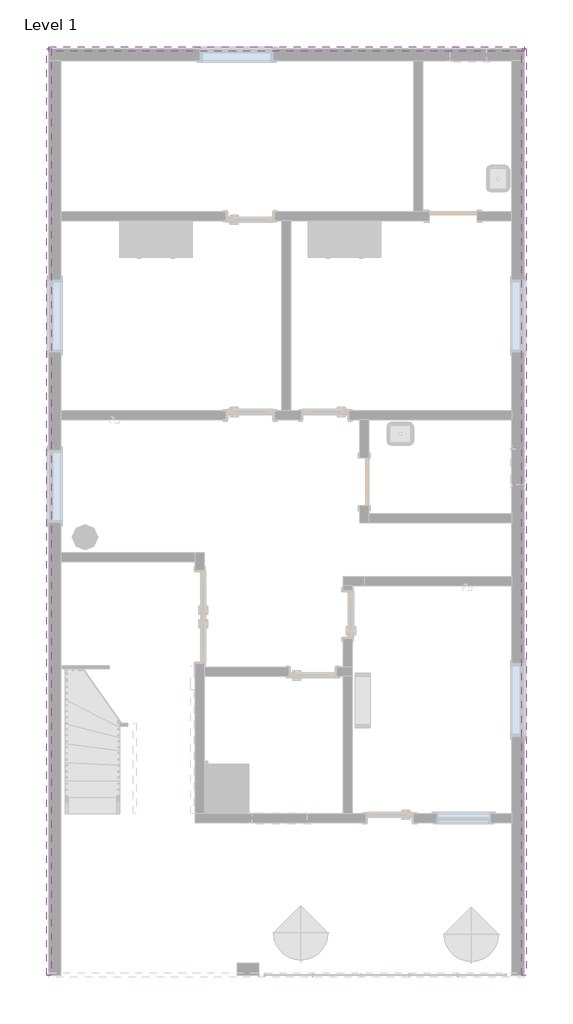
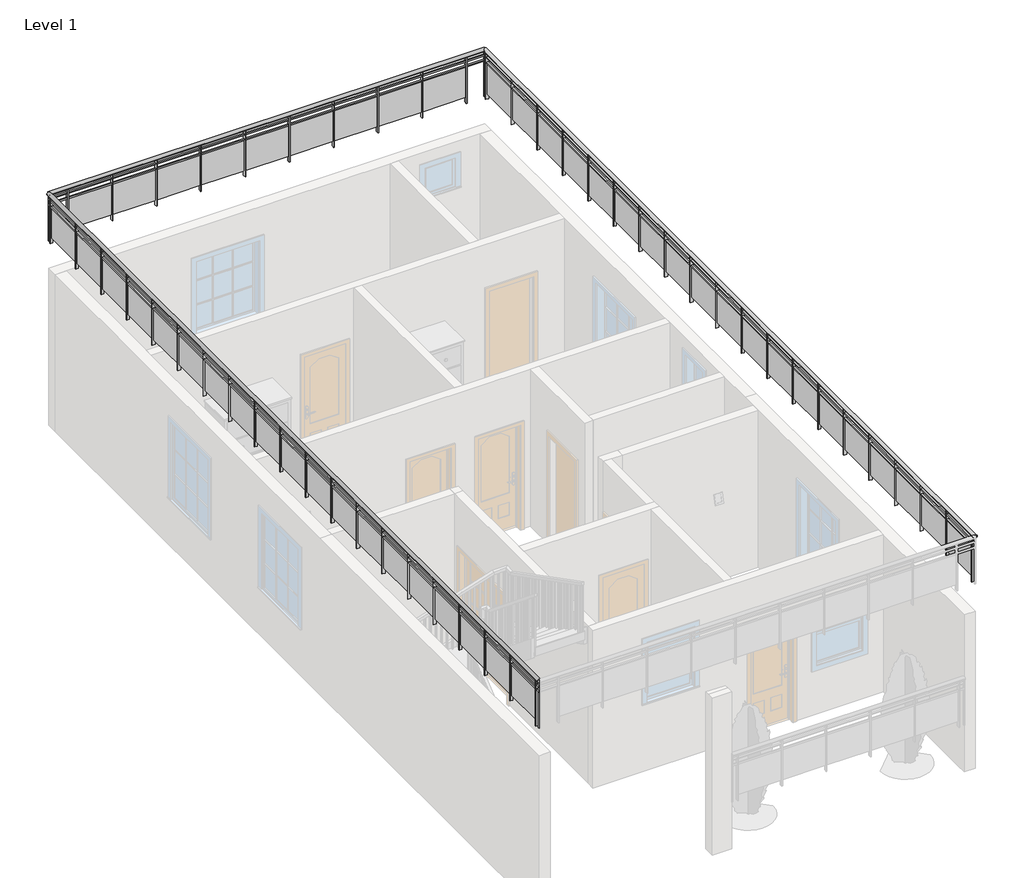
# One storey, part 3 of 4: 3 railings.
"""IFC4 building model written with IfcOpenShell, lengths in millimetres."""

from ifc_helpers import new_model, si_unit, point, frame, origin, place, context, project, spatial, polyline, ellipse_curve, trimmed, outline, extrude, element, save
from ifc_brep_helpers import plane_surface, extruded_surface, advanced_brep

model = new_model("IFC4")

# Units and contexts
model_context = context("Model", 3, world=origin())
ifc_project = project(units=[si_unit("LENGTHUNIT", "METRE", prefix="MILLI")], contexts=[model_context])

# Site, building, storey
site = spatial("IfcSite", under=ifc_project)
building = spatial("IfcBuilding", under=site)
storey = spatial("IfcBuildingStorey", under=building, Name="Level 1", Elevation=0.0)

# Railings
placement = place(None, origin())
element("IfcRailing", 1, ObjectType="Glass Panel - Bottom Fill", at=placement, inside=storey, context=model_context, shape_type="SolidModel", body=[
    advanced_brep(
    [(-13526.4568901, 13670.121124, 4495.8), (-13602.6568901, 13670.121124, 4495.8), (-13526.4568901, -1925.478876, 4495.8), (-13602.6568901, -1925.478876, 4495.8)],
    [
        (0, 1, ellipse_curve(frame((-13564.5568901, 13670.121124, 4495.8), z_axis=(0.0, 1.0, 0.0), x_axis=(-1.0, 0.0, 0.0)), 38.1, 28.575)),
        (1, 0, ellipse_curve(frame((-13564.5568901, 13670.121124, 4495.8), z_axis=(0.0, 1.0, 0.0), x_axis=(-1.0, 0.0, 0.0)), 38.1, 28.575)),
        (2, 3, ellipse_curve(frame((-13564.5568901, -1925.478876, 4495.8), z_axis=(0.0, -1.0, 0.0), x_axis=(-1.0, 0.0, 0.0)), 38.1, 28.575)),
        (3, 2, ellipse_curve(frame((-13564.5568901, -1925.478876, 4495.8), z_axis=(0.0, -1.0, 0.0), x_axis=(-1.0, 0.0, 0.0)), 38.1, 28.575)),
        (0, 2),
        (3, 1),
    ],
    [
        plane_surface(frame((-13564.5568901, 13670.121124, 4495.8), z_axis=(0.0, 1.0, 0.0), x_axis=(0.0, 0.0, -1.0))),
        plane_surface(frame((-13564.5568901, -1925.478876, 4495.8), z_axis=(0.0, -1.0, 0.0), x_axis=(0.0, 0.0, -1.0))),
        extruded_surface(trimmed(ellipse_curve(frame((-13564.5568901, -1925.478876, 4495.8), z_axis=(0.0, 1.0, 0.0), x_axis=(-1.0, 0.0, 0.0)), 38.1, 28.575), [point((-13526.4568901, -1925.478876, 4495.8))], [point((-13602.6568901, -1925.478876, 4495.8))], True, "CARTESIAN"), (0.0, 15595.599999999999, 0.0), 15595.599999999999),
        extruded_surface(trimmed(ellipse_curve(frame((-13564.5568901, -1925.478876, 4495.8), z_axis=(0.0, 1.0, 0.0), x_axis=(-1.0, 0.0, 0.0)), 38.1, 28.575), [point((-13602.6568901, -1925.478876, 4495.8))], [point((-13526.4568901, -1925.478876, 4495.8))], True, "CARTESIAN"), (0.0, 15595.599999999999, 0.0), 15595.599999999999),
    ],
    [
        (0, [[1, 2]]),
        (1, [[3, 4]]),
        (2, [[-1, 5, -4, 6]]),
        (3, [[-2, -6, -3, -5]]),
    ],
),
    extrude(outline(polyline([(-13577.2568901, 13670.121124), (-13551.8568901, 13670.121124), (-13551.8568901, -1925.478876), (-13577.2568901, -1925.478876), (-13577.2568901, 13670.121124)])), frame((0.0, 0.0, 4381.5), z_axis=(0.0, 0.0, 1.0), x_axis=(1.0, 0.0, 0.0)), (0.0, 0.0, 1.0), 25.4),
    extrude(outline(polyline([(-13577.2568901, 13670.121124), (-13551.8568901, 13670.121124), (-13551.8568901, -1925.478876), (-13577.2568901, -1925.478876), (-13577.2568901, 13670.121124)])), frame((0.0, 0.0, 4279.9), z_axis=(0.0, 0.0, 1.0), x_axis=(1.0, 0.0, 0.0)), (0.0, 0.0, 1.0), 25.4),
    extrude(outline(polyline([(-13589.9568901, -1842.928876), (-13539.1568901, -1842.928876), (-13539.1568901, -1855.628876), (-13589.9568901, -1855.628876), (-13589.9568901, -1842.928876)])), frame((0.0, 0.0, 3581.4), z_axis=(0.0, 0.0, 1.0), x_axis=(1.0, 0.0, 0.0)), (0.0, 0.0, 1.0), 885.6788223),
    extrude(outline(polyline([(-13558.0217331, -1036.478876), (-13558.0217331, -1849.278876), (-13564.3717331, -1849.278876), (-13564.3717331, -1036.478876), (-13558.0217331, -1036.478876)])), frame((0.0, 0.0, 3683.0), z_axis=(0.0, 0.0, 1.0), x_axis=(1.0, 0.0, 0.0)), (0.0, 0.0, 1.0), 596.9),
    extrude(outline(polyline([(-13589.9568901, -1030.128876), (-13539.1568901, -1030.128876), (-13539.1568901, -1042.828876), (-13589.9568901, -1042.828876), (-13589.9568901, -1030.128876)])), frame((0.0, 0.0, 3581.4), z_axis=(0.0, 0.0, 1.0), x_axis=(1.0, 0.0, 0.0)), (0.0, 0.0, 1.0), 885.6788223),
    extrude(outline(polyline([(-13558.0217331, -223.678876), (-13558.0217331, -1036.478876), (-13564.3717331, -1036.478876), (-13564.3717331, -223.678876), (-13558.0217331, -223.678876)])), frame((0.0, 0.0, 3683.0), z_axis=(0.0, 0.0, 1.0), x_axis=(1.0, 0.0, 0.0)), (0.0, 0.0, 1.0), 596.9),
    extrude(outline(polyline([(-13589.9568901, -217.328876), (-13539.1568901, -217.328876), (-13539.1568901, -230.028876), (-13589.9568901, -230.028876), (-13589.9568901, -217.328876)])), frame((0.0, 0.0, 3581.4), z_axis=(0.0, 0.0, 1.0), x_axis=(1.0, 0.0, 0.0)), (0.0, 0.0, 1.0), 885.6788223),
    extrude(outline(polyline([(-13558.0217331, 589.121124), (-13558.0217331, -223.678876), (-13564.3717331, -223.678876), (-13564.3717331, 589.121124), (-13558.0217331, 589.121124)])), frame((0.0, 0.0, 3683.0), z_axis=(0.0, 0.0, 1.0), x_axis=(1.0, 0.0, 0.0)), (0.0, 0.0, 1.0), 596.9),
    extrude(outline(polyline([(-13589.9568901, 595.471124), (-13539.1568901, 595.471124), (-13539.1568901, 582.771124), (-13589.9568901, 582.771124), (-13589.9568901, 595.471124)])), frame((0.0, 0.0, 3581.4), z_axis=(0.0, 0.0, 1.0), x_axis=(1.0, 0.0, 0.0)), (0.0, 0.0, 1.0), 885.6788223),
    extrude(outline(polyline([(-13558.0217331, 1401.921124), (-13558.0217331, 589.121124), (-13564.3717331, 589.121124), (-13564.3717331, 1401.921124), (-13558.0217331, 1401.921124)])), frame((0.0, 0.0, 3683.0), z_axis=(0.0, 0.0, 1.0), x_axis=(1.0, 0.0, 0.0)), (0.0, 0.0, 1.0), 596.9),
    extrude(outline(polyline([(-13589.9568901, 1408.271124), (-13539.1568901, 1408.271124), (-13539.1568901, 1395.571124), (-13589.9568901, 1395.571124), (-13589.9568901, 1408.271124)])), frame((0.0, 0.0, 3581.4), z_axis=(0.0, 0.0, 1.0), x_axis=(1.0, 0.0, 0.0)), (0.0, 0.0, 1.0), 885.6788223),
    extrude(outline(polyline([(-13558.0217331, 2214.721124), (-13558.0217331, 1401.921124), (-13564.3717331, 1401.921124), (-13564.3717331, 2214.721124), (-13558.0217331, 2214.721124)])), frame((0.0, 0.0, 3683.0), z_axis=(0.0, 0.0, 1.0), x_axis=(1.0, 0.0, 0.0)), (0.0, 0.0, 1.0), 596.9),
    extrude(outline(polyline([(-13589.9568901, 2221.071124), (-13539.1568901, 2221.071124), (-13539.1568901, 2208.371124), (-13589.9568901, 2208.371124), (-13589.9568901, 2221.071124)])), frame((0.0, 0.0, 3581.4), z_axis=(0.0, 0.0, 1.0), x_axis=(1.0, 0.0, 0.0)), (0.0, 0.0, 1.0), 885.6788223),
    extrude(outline(polyline([(-13558.0217331, 3027.521124), (-13558.0217331, 2214.721124), (-13564.3717331, 2214.721124), (-13564.3717331, 3027.521124), (-13558.0217331, 3027.521124)])), frame((0.0, 0.0, 3683.0), z_axis=(0.0, 0.0, 1.0), x_axis=(1.0, 0.0, 0.0)), (0.0, 0.0, 1.0), 596.9),
    extrude(outline(polyline([(-13589.9568901, 3033.871124), (-13539.1568901, 3033.871124), (-13539.1568901, 3021.171124), (-13589.9568901, 3021.171124), (-13589.9568901, 3033.871124)])), frame((0.0, 0.0, 3581.4), z_axis=(0.0, 0.0, 1.0), x_axis=(1.0, 0.0, 0.0)), (0.0, 0.0, 1.0), 885.6788223),
    extrude(outline(polyline([(-13558.0217331, 3840.321124), (-13558.0217331, 3027.521124), (-13564.3717331, 3027.521124), (-13564.3717331, 3840.321124), (-13558.0217331, 3840.321124)])), frame((0.0, 0.0, 3683.0), z_axis=(0.0, 0.0, 1.0), x_axis=(1.0, 0.0, 0.0)), (0.0, 0.0, 1.0), 596.9),
    extrude(outline(polyline([(-13589.9568901, 3846.671124), (-13539.1568901, 3846.671124), (-13539.1568901, 3833.971124), (-13589.9568901, 3833.971124), (-13589.9568901, 3846.671124)])), frame((0.0, 0.0, 3581.4), z_axis=(0.0, 0.0, 1.0), x_axis=(1.0, 0.0, 0.0)), (0.0, 0.0, 1.0), 885.6788223),
    extrude(outline(polyline([(-13558.0217331, 4653.121124), (-13558.0217331, 3840.321124), (-13564.3717331, 3840.321124), (-13564.3717331, 4653.121124), (-13558.0217331, 4653.121124)])), frame((0.0, 0.0, 3683.0), z_axis=(0.0, 0.0, 1.0), x_axis=(1.0, 0.0, 0.0)), (0.0, 0.0, 1.0), 596.9),
    extrude(outline(polyline([(-13589.9568901, 4659.471124), (-13539.1568901, 4659.471124), (-13539.1568901, 4646.771124), (-13589.9568901, 4646.771124), (-13589.9568901, 4659.471124)])), frame((0.0, 0.0, 3581.4), z_axis=(0.0, 0.0, 1.0), x_axis=(1.0, 0.0, 0.0)), (0.0, 0.0, 1.0), 885.6788223),
    extrude(outline(polyline([(-13558.0217331, 5465.921124), (-13558.0217331, 4653.121124), (-13564.3717331, 4653.121124), (-13564.3717331, 5465.921124), (-13558.0217331, 5465.921124)])), frame((0.0, 0.0, 3683.0), z_axis=(0.0, 0.0, 1.0), x_axis=(1.0, 0.0, 0.0)), (0.0, 0.0, 1.0), 596.9),
    extrude(outline(polyline([(-13589.9568901, 5472.271124), (-13539.1568901, 5472.271124), (-13539.1568901, 5459.571124), (-13589.9568901, 5459.571124), (-13589.9568901, 5472.271124)])), frame((0.0, 0.0, 3581.4), z_axis=(0.0, 0.0, 1.0), x_axis=(1.0, 0.0, 0.0)), (0.0, 0.0, 1.0), 885.6788223),
    extrude(outline(polyline([(-13558.0217331, 6278.721124), (-13558.0217331, 5465.921124), (-13564.3717331, 5465.921124), (-13564.3717331, 6278.721124), (-13558.0217331, 6278.721124)])), frame((0.0, 0.0, 3683.0), z_axis=(0.0, 0.0, 1.0), x_axis=(1.0, 0.0, 0.0)), (0.0, 0.0, 1.0), 596.9),
    extrude(outline(polyline([(-13589.9568901, 6285.071124), (-13539.1568901, 6285.071124), (-13539.1568901, 6272.371124), (-13589.9568901, 6272.371124), (-13589.9568901, 6285.071124)])), frame((0.0, 0.0, 3581.4), z_axis=(0.0, 0.0, 1.0), x_axis=(1.0, 0.0, 0.0)), (0.0, 0.0, 1.0), 885.6788223),
    extrude(outline(polyline([(-13558.0217331, 7091.521124), (-13558.0217331, 6278.721124), (-13564.3717331, 6278.721124), (-13564.3717331, 7091.521124), (-13558.0217331, 7091.521124)])), frame((0.0, 0.0, 3683.0), z_axis=(0.0, 0.0, 1.0), x_axis=(1.0, 0.0, 0.0)), (0.0, 0.0, 1.0), 596.9),
    extrude(outline(polyline([(-13589.9568901, 7097.871124), (-13539.1568901, 7097.871124), (-13539.1568901, 7085.171124), (-13589.9568901, 7085.171124), (-13589.9568901, 7097.871124)])), frame((0.0, 0.0, 3581.4), z_axis=(0.0, 0.0, 1.0), x_axis=(1.0, 0.0, 0.0)), (0.0, 0.0, 1.0), 885.6788223),
    extrude(outline(polyline([(-13558.0217331, 7904.321124), (-13558.0217331, 7091.521124), (-13564.3717331, 7091.521124), (-13564.3717331, 7904.321124), (-13558.0217331, 7904.321124)])), frame((0.0, 0.0, 3683.0), z_axis=(0.0, 0.0, 1.0), x_axis=(1.0, 0.0, 0.0)), (0.0, 0.0, 1.0), 596.9),
    extrude(outline(polyline([(-13589.9568901, 7910.671124), (-13539.1568901, 7910.671124), (-13539.1568901, 7897.971124), (-13589.9568901, 7897.971124), (-13589.9568901, 7910.671124)])), frame((0.0, 0.0, 3581.4), z_axis=(0.0, 0.0, 1.0), x_axis=(1.0, 0.0, 0.0)), (0.0, 0.0, 1.0), 885.6788223),
    extrude(outline(polyline([(-13558.0217331, 8717.121124), (-13558.0217331, 7904.321124), (-13564.3717331, 7904.321124), (-13564.3717331, 8717.121124), (-13558.0217331, 8717.121124)])), frame((0.0, 0.0, 3683.0), z_axis=(0.0, 0.0, 1.0), x_axis=(1.0, 0.0, 0.0)), (0.0, 0.0, 1.0), 596.9),
    extrude(outline(polyline([(-13589.9568901, 8723.471124), (-13539.1568901, 8723.471124), (-13539.1568901, 8710.771124), (-13589.9568901, 8710.771124), (-13589.9568901, 8723.471124)])), frame((0.0, 0.0, 3581.4), z_axis=(0.0, 0.0, 1.0), x_axis=(1.0, 0.0, 0.0)), (0.0, 0.0, 1.0), 885.6788223),
    extrude(outline(polyline([(-13558.0217331, 9529.921124), (-13558.0217331, 8717.121124), (-13564.3717331, 8717.121124), (-13564.3717331, 9529.921124), (-13558.0217331, 9529.921124)])), frame((0.0, 0.0, 3683.0), z_axis=(0.0, 0.0, 1.0), x_axis=(1.0, 0.0, 0.0)), (0.0, 0.0, 1.0), 596.9),
    extrude(outline(polyline([(-13589.9568901, 9536.271124), (-13539.1568901, 9536.271124), (-13539.1568901, 9523.571124), (-13589.9568901, 9523.571124), (-13589.9568901, 9536.271124)])), frame((0.0, 0.0, 3581.4), z_axis=(0.0, 0.0, 1.0), x_axis=(1.0, 0.0, 0.0)), (0.0, 0.0, 1.0), 885.6788223),
    extrude(outline(polyline([(-13558.0217331, 10342.721124), (-13558.0217331, 9529.921124), (-13564.3717331, 9529.921124), (-13564.3717331, 10342.721124), (-13558.0217331, 10342.721124)])), frame((0.0, 0.0, 3683.0), z_axis=(0.0, 0.0, 1.0), x_axis=(1.0, 0.0, 0.0)), (0.0, 0.0, 1.0), 596.9),
    extrude(outline(polyline([(-13589.9568901, 10349.071124), (-13539.1568901, 10349.071124), (-13539.1568901, 10336.371124), (-13589.9568901, 10336.371124), (-13589.9568901, 10349.071124)])), frame((0.0, 0.0, 3581.4), z_axis=(0.0, 0.0, 1.0), x_axis=(1.0, 0.0, 0.0)), (0.0, 0.0, 1.0), 885.6788223),
    extrude(outline(polyline([(-13558.0217331, 11155.521124), (-13558.0217331, 10342.721124), (-13564.3717331, 10342.721124), (-13564.3717331, 11155.521124), (-13558.0217331, 11155.521124)])), frame((0.0, 0.0, 3683.0), z_axis=(0.0, 0.0, 1.0), x_axis=(1.0, 0.0, 0.0)), (0.0, 0.0, 1.0), 596.9),
    extrude(outline(polyline([(-13589.9568901, 11161.871124), (-13539.1568901, 11161.871124), (-13539.1568901, 11149.171124), (-13589.9568901, 11149.171124), (-13589.9568901, 11161.871124)])), frame((0.0, 0.0, 3581.4), z_axis=(0.0, 0.0, 1.0), x_axis=(1.0, 0.0, 0.0)), (0.0, 0.0, 1.0), 885.6788223),
    extrude(outline(polyline([(-13558.0217331, 11968.321124), (-13558.0217331, 11155.521124), (-13564.3717331, 11155.521124), (-13564.3717331, 11968.321124), (-13558.0217331, 11968.321124)])), frame((0.0, 0.0, 3683.0), z_axis=(0.0, 0.0, 1.0), x_axis=(1.0, 0.0, 0.0)), (0.0, 0.0, 1.0), 596.9),
    extrude(outline(polyline([(-13589.9568901, 11974.671124), (-13539.1568901, 11974.671124), (-13539.1568901, 11961.971124), (-13589.9568901, 11961.971124), (-13589.9568901, 11974.671124)])), frame((0.0, 0.0, 3581.4), z_axis=(0.0, 0.0, 1.0), x_axis=(1.0, 0.0, 0.0)), (0.0, 0.0, 1.0), 885.6788223),
    extrude(outline(polyline([(-13558.0217331, 12781.121124), (-13558.0217331, 11968.321124), (-13564.3717331, 11968.321124), (-13564.3717331, 12781.121124), (-13558.0217331, 12781.121124)])), frame((0.0, 0.0, 3683.0), z_axis=(0.0, 0.0, 1.0), x_axis=(1.0, 0.0, 0.0)), (0.0, 0.0, 1.0), 596.9),
    extrude(outline(polyline([(-13589.9568901, 12787.471124), (-13539.1568901, 12787.471124), (-13539.1568901, 12774.771124), (-13589.9568901, 12774.771124), (-13589.9568901, 12787.471124)])), frame((0.0, 0.0, 3581.4), z_axis=(0.0, 0.0, 1.0), x_axis=(1.0, 0.0, 0.0)), (0.0, 0.0, 1.0), 885.6788223),
    extrude(outline(polyline([(-13558.0217331, 13593.921124), (-13558.0217331, 12781.121124), (-13564.3717331, 12781.121124), (-13564.3717331, 13593.921124), (-13558.0217331, 13593.921124)])), frame((0.0, 0.0, 3683.0), z_axis=(0.0, 0.0, 1.0), x_axis=(1.0, 0.0, 0.0)), (0.0, 0.0, 1.0), 596.9),
    extrude(outline(polyline([(-13589.9568901, 13600.271124), (-13539.1568901, 13600.271124), (-13539.1568901, 13587.571124), (-13589.9568901, 13587.571124), (-13589.9568901, 13600.271124)])), frame((0.0, 0.0, 3581.4), z_axis=(0.0, 0.0, 1.0), x_axis=(1.0, 0.0, 0.0)), (0.0, 0.0, 1.0), 885.6788223),
    extrude(outline(polyline([(-13574.0818901, -1912.778876), (-13555.0318901, -1912.778876), (-13555.0318901, -1931.828876), (-13574.0818901, -1931.828876), (-13574.0818901, -1912.778876)])), frame((0.0, 0.0, 3581.4), z_axis=(0.0, 0.0, 1.0), x_axis=(1.0, 0.0, 0.0)), (0.0, 0.0, 1.0), 885.6788223),
    extrude(outline(polyline([(-13574.0818901, 13676.471124), (-13555.0318901, 13676.471124), (-13555.0318901, 13657.421124), (-13574.0818901, 13657.421124), (-13574.0818901, 13676.471124)])), frame((0.0, 0.0, 3581.4), z_axis=(0.0, 0.0, 1.0), x_axis=(1.0, 0.0, 0.0)), (0.0, 0.0, 1.0), 885.6788223),
])
element("IfcRailing", 2, ObjectType="Glass Panel - Bottom Fill", at=placement, inside=storey, context=model_context, shape_type="SolidModel", body=[
    advanced_brep(
    [(-5601.6568901, -1925.478876, 4495.8), (-5525.4568901, -1925.478876, 4495.8), (-5601.6568901, 13670.121124, 4495.8), (-5525.4568901, 13670.121124, 4495.8)],
    [
        (0, 1, ellipse_curve(frame((-5563.5568901, -1925.478876, 4495.8), z_axis=(0.0, -1.0, 0.0), x_axis=(1.0, 0.0, 0.0)), 38.1, 28.575)),
        (1, 0, ellipse_curve(frame((-5563.5568901, -1925.478876, 4495.8), z_axis=(0.0, -1.0, 0.0), x_axis=(1.0, 0.0, 0.0)), 38.1, 28.575)),
        (2, 3, ellipse_curve(frame((-5563.5568901, 13670.121124, 4495.8), z_axis=(0.0, 1.0, 0.0), x_axis=(1.0, 0.0, 0.0)), 38.1, 28.575)),
        (3, 2, ellipse_curve(frame((-5563.5568901, 13670.121124, 4495.8), z_axis=(0.0, 1.0, 0.0), x_axis=(1.0, 0.0, 0.0)), 38.1, 28.575)),
        (0, 2),
        (3, 1),
    ],
    [
        plane_surface(frame((-5563.5568901, -1925.478876, 4495.8), z_axis=(0.0, -1.0, 0.0), x_axis=(0.0, 0.0, 1.0))),
        plane_surface(frame((-5563.5568901, 13670.121124, 4495.8), z_axis=(0.0, 1.0, 0.0), x_axis=(0.0, 0.0, 1.0))),
        extruded_surface(trimmed(ellipse_curve(frame((-5563.5568901, 13670.121124, 4495.8), z_axis=(0.0, -1.0, 0.0), x_axis=(1.0, 0.0, 0.0)), 38.1, 28.575), [point((-5601.6568901, 13670.121124, 4495.8))], [point((-5525.4568901, 13670.121124, 4495.8))], True, "CARTESIAN"), (0.0, -15595.599999999999, 0.0), 15595.599999999999),
        extruded_surface(trimmed(ellipse_curve(frame((-5563.5568901, 13670.121124, 4495.8), z_axis=(0.0, -1.0, 0.0), x_axis=(1.0, 0.0, 0.0)), 38.1, 28.575), [point((-5525.4568901, 13670.121124, 4495.8))], [point((-5601.6568901, 13670.121124, 4495.8))], True, "CARTESIAN"), (0.0, -15595.599999999999, 0.0), 15595.599999999999),
    ],
    [
        (0, [[1, 2]]),
        (1, [[3, 4]]),
        (2, [[-1, 5, -4, 6]]),
        (3, [[-2, -6, -3, -5]]),
    ],
),
    extrude(outline(polyline([(-5550.8568901, -1925.478876), (-5576.2568901, -1925.478876), (-5576.2568901, 13670.121124), (-5550.8568901, 13670.121124), (-5550.8568901, -1925.478876)])), frame((0.0, 0.0, 4381.5), z_axis=(0.0, 0.0, 1.0), x_axis=(1.0, 0.0, 0.0)), (0.0, 0.0, 1.0), 25.4),
    extrude(outline(polyline([(-5550.8568901, -1925.478876), (-5576.2568901, -1925.478876), (-5576.2568901, 13670.121124), (-5550.8568901, 13670.121124), (-5550.8568901, -1925.478876)])), frame((0.0, 0.0, 4279.9), z_axis=(0.0, 0.0, 1.0), x_axis=(1.0, 0.0, 0.0)), (0.0, 0.0, 1.0), 25.4),
    extrude(outline(polyline([(-5538.1568901, 13587.571124), (-5588.9568901, 13587.571124), (-5588.9568901, 13600.271124), (-5538.1568901, 13600.271124), (-5538.1568901, 13587.571124)])), frame((0.0, 0.0, 3581.4), z_axis=(0.0, 0.0, 1.0), x_axis=(1.0, 0.0, 0.0)), (0.0, 0.0, 1.0), 885.6788223),
    extrude(outline(polyline([(-5570.0920471, 12781.121124), (-5570.0920471, 13593.921124), (-5563.7420471, 13593.921124), (-5563.7420471, 12781.121124), (-5570.0920471, 12781.121124)])), frame((0.0, 0.0, 3683.0), z_axis=(0.0, 0.0, 1.0), x_axis=(1.0, 0.0, 0.0)), (0.0, 0.0, 1.0), 596.9),
    extrude(outline(polyline([(-5538.1568901, 12774.771124), (-5588.9568901, 12774.771124), (-5588.9568901, 12787.471124), (-5538.1568901, 12787.471124), (-5538.1568901, 12774.771124)])), frame((0.0, 0.0, 3581.4), z_axis=(0.0, 0.0, 1.0), x_axis=(1.0, 0.0, 0.0)), (0.0, 0.0, 1.0), 885.6788223),
    extrude(outline(polyline([(-5570.0920471, 11968.321124), (-5570.0920471, 12781.121124), (-5563.7420471, 12781.121124), (-5563.7420471, 11968.321124), (-5570.0920471, 11968.321124)])), frame((0.0, 0.0, 3683.0), z_axis=(0.0, 0.0, 1.0), x_axis=(1.0, 0.0, 0.0)), (0.0, 0.0, 1.0), 596.9),
    extrude(outline(polyline([(-5538.1568901, 11961.971124), (-5588.9568901, 11961.971124), (-5588.9568901, 11974.671124), (-5538.1568901, 11974.671124), (-5538.1568901, 11961.971124)])), frame((0.0, 0.0, 3581.4), z_axis=(0.0, 0.0, 1.0), x_axis=(1.0, 0.0, 0.0)), (0.0, 0.0, 1.0), 885.6788223),
    extrude(outline(polyline([(-5570.0920471, 11155.521124), (-5570.0920471, 11968.321124), (-5563.7420471, 11968.321124), (-5563.7420471, 11155.521124), (-5570.0920471, 11155.521124)])), frame((0.0, 0.0, 3683.0), z_axis=(0.0, 0.0, 1.0), x_axis=(1.0, 0.0, 0.0)), (0.0, 0.0, 1.0), 596.9),
    extrude(outline(polyline([(-5538.1568901, 11149.171124), (-5588.9568901, 11149.171124), (-5588.9568901, 11161.871124), (-5538.1568901, 11161.871124), (-5538.1568901, 11149.171124)])), frame((0.0, 0.0, 3581.4), z_axis=(0.0, 0.0, 1.0), x_axis=(1.0, 0.0, 0.0)), (0.0, 0.0, 1.0), 885.6788223),
    extrude(outline(polyline([(-5570.0920471, 10342.721124), (-5570.0920471, 11155.521124), (-5563.7420471, 11155.521124), (-5563.7420471, 10342.721124), (-5570.0920471, 10342.721124)])), frame((0.0, 0.0, 3683.0), z_axis=(0.0, 0.0, 1.0), x_axis=(1.0, 0.0, 0.0)), (0.0, 0.0, 1.0), 596.9),
    extrude(outline(polyline([(-5538.1568901, 10336.371124), (-5588.9568901, 10336.371124), (-5588.9568901, 10349.071124), (-5538.1568901, 10349.071124), (-5538.1568901, 10336.371124)])), frame((0.0, 0.0, 3581.4), z_axis=(0.0, 0.0, 1.0), x_axis=(1.0, 0.0, 0.0)), (0.0, 0.0, 1.0), 885.6788223),
    extrude(outline(polyline([(-5570.0920471, 9529.921124), (-5570.0920471, 10342.721124), (-5563.7420471, 10342.721124), (-5563.7420471, 9529.921124), (-5570.0920471, 9529.921124)])), frame((0.0, 0.0, 3683.0), z_axis=(0.0, 0.0, 1.0), x_axis=(1.0, 0.0, 0.0)), (0.0, 0.0, 1.0), 596.9),
    extrude(outline(polyline([(-5538.1568901, 9523.571124), (-5588.9568901, 9523.571124), (-5588.9568901, 9536.271124), (-5538.1568901, 9536.271124), (-5538.1568901, 9523.571124)])), frame((0.0, 0.0, 3581.4), z_axis=(0.0, 0.0, 1.0), x_axis=(1.0, 0.0, 0.0)), (0.0, 0.0, 1.0), 885.6788223),
    extrude(outline(polyline([(-5570.0920471, 8717.121124), (-5570.0920471, 9529.921124), (-5563.7420471, 9529.921124), (-5563.7420471, 8717.121124), (-5570.0920471, 8717.121124)])), frame((0.0, 0.0, 3683.0), z_axis=(0.0, 0.0, 1.0), x_axis=(1.0, 0.0, 0.0)), (0.0, 0.0, 1.0), 596.9),
    extrude(outline(polyline([(-5538.1568901, 8710.771124), (-5588.9568901, 8710.771124), (-5588.9568901, 8723.471124), (-5538.1568901, 8723.471124), (-5538.1568901, 8710.771124)])), frame((0.0, 0.0, 3581.4), z_axis=(0.0, 0.0, 1.0), x_axis=(1.0, 0.0, 0.0)), (0.0, 0.0, 1.0), 885.6788223),
    extrude(outline(polyline([(-5570.0920471, 7904.321124), (-5570.0920471, 8717.121124), (-5563.7420471, 8717.121124), (-5563.7420471, 7904.321124), (-5570.0920471, 7904.321124)])), frame((0.0, 0.0, 3683.0), z_axis=(0.0, 0.0, 1.0), x_axis=(1.0, 0.0, 0.0)), (0.0, 0.0, 1.0), 596.9),
    extrude(outline(polyline([(-5538.1568901, 7897.971124), (-5588.9568901, 7897.971124), (-5588.9568901, 7910.671124), (-5538.1568901, 7910.671124), (-5538.1568901, 7897.971124)])), frame((0.0, 0.0, 3581.4), z_axis=(0.0, 0.0, 1.0), x_axis=(1.0, 0.0, 0.0)), (0.0, 0.0, 1.0), 885.6788223),
    extrude(outline(polyline([(-5570.0920471, 7091.521124), (-5570.0920471, 7904.321124), (-5563.7420471, 7904.321124), (-5563.7420471, 7091.521124), (-5570.0920471, 7091.521124)])), frame((0.0, 0.0, 3683.0), z_axis=(0.0, 0.0, 1.0), x_axis=(1.0, 0.0, 0.0)), (0.0, 0.0, 1.0), 596.9),
    extrude(outline(polyline([(-5538.1568901, 7085.171124), (-5588.9568901, 7085.171124), (-5588.9568901, 7097.871124), (-5538.1568901, 7097.871124), (-5538.1568901, 7085.171124)])), frame((0.0, 0.0, 3581.4), z_axis=(0.0, 0.0, 1.0), x_axis=(1.0, 0.0, 0.0)), (0.0, 0.0, 1.0), 885.6788223),
    extrude(outline(polyline([(-5570.0920471, 6278.721124), (-5570.0920471, 7091.521124), (-5563.7420471, 7091.521124), (-5563.7420471, 6278.721124), (-5570.0920471, 6278.721124)])), frame((0.0, 0.0, 3683.0), z_axis=(0.0, 0.0, 1.0), x_axis=(1.0, 0.0, 0.0)), (0.0, 0.0, 1.0), 596.9),
    extrude(outline(polyline([(-5538.1568901, 6272.371124), (-5588.9568901, 6272.371124), (-5588.9568901, 6285.071124), (-5538.1568901, 6285.071124), (-5538.1568901, 6272.371124)])), frame((0.0, 0.0, 3581.4), z_axis=(0.0, 0.0, 1.0), x_axis=(1.0, 0.0, 0.0)), (0.0, 0.0, 1.0), 885.6788223),
    extrude(outline(polyline([(-5570.0920471, 5465.921124), (-5570.0920471, 6278.721124), (-5563.7420471, 6278.721124), (-5563.7420471, 5465.921124), (-5570.0920471, 5465.921124)])), frame((0.0, 0.0, 3683.0), z_axis=(0.0, 0.0, 1.0), x_axis=(1.0, 0.0, 0.0)), (0.0, 0.0, 1.0), 596.9),
    extrude(outline(polyline([(-5538.1568901, 5459.571124), (-5588.9568901, 5459.571124), (-5588.9568901, 5472.271124), (-5538.1568901, 5472.271124), (-5538.1568901, 5459.571124)])), frame((0.0, 0.0, 3581.4), z_axis=(0.0, 0.0, 1.0), x_axis=(1.0, 0.0, 0.0)), (0.0, 0.0, 1.0), 885.6788223),
    extrude(outline(polyline([(-5570.0920471, 4653.121124), (-5570.0920471, 5465.921124), (-5563.7420471, 5465.921124), (-5563.7420471, 4653.121124), (-5570.0920471, 4653.121124)])), frame((0.0, 0.0, 3683.0), z_axis=(0.0, 0.0, 1.0), x_axis=(1.0, 0.0, 0.0)), (0.0, 0.0, 1.0), 596.9),
    extrude(outline(polyline([(-5538.1568901, 4646.771124), (-5588.9568901, 4646.771124), (-5588.9568901, 4659.471124), (-5538.1568901, 4659.471124), (-5538.1568901, 4646.771124)])), frame((0.0, 0.0, 3581.4), z_axis=(0.0, 0.0, 1.0), x_axis=(1.0, 0.0, 0.0)), (0.0, 0.0, 1.0), 885.6788223),
    extrude(outline(polyline([(-5570.0920471, 3840.321124), (-5570.0920471, 4653.121124), (-5563.7420471, 4653.121124), (-5563.7420471, 3840.321124), (-5570.0920471, 3840.321124)])), frame((0.0, 0.0, 3683.0), z_axis=(0.0, 0.0, 1.0), x_axis=(1.0, 0.0, 0.0)), (0.0, 0.0, 1.0), 596.9),
    extrude(outline(polyline([(-5538.1568901, 3833.971124), (-5588.9568901, 3833.971124), (-5588.9568901, 3846.671124), (-5538.1568901, 3846.671124), (-5538.1568901, 3833.971124)])), frame((0.0, 0.0, 3581.4), z_axis=(0.0, 0.0, 1.0), x_axis=(1.0, 0.0, 0.0)), (0.0, 0.0, 1.0), 885.6788223),
    extrude(outline(polyline([(-5570.0920471, 3027.521124), (-5570.0920471, 3840.321124), (-5563.7420471, 3840.321124), (-5563.7420471, 3027.521124), (-5570.0920471, 3027.521124)])), frame((0.0, 0.0, 3683.0), z_axis=(0.0, 0.0, 1.0), x_axis=(1.0, 0.0, 0.0)), (0.0, 0.0, 1.0), 596.9),
    extrude(outline(polyline([(-5538.1568901, 3021.171124), (-5588.9568901, 3021.171124), (-5588.9568901, 3033.871124), (-5538.1568901, 3033.871124), (-5538.1568901, 3021.171124)])), frame((0.0, 0.0, 3581.4), z_axis=(0.0, 0.0, 1.0), x_axis=(1.0, 0.0, 0.0)), (0.0, 0.0, 1.0), 885.6788223),
    extrude(outline(polyline([(-5570.0920471, 2214.721124), (-5570.0920471, 3027.521124), (-5563.7420471, 3027.521124), (-5563.7420471, 2214.721124), (-5570.0920471, 2214.721124)])), frame((0.0, 0.0, 3683.0), z_axis=(0.0, 0.0, 1.0), x_axis=(1.0, 0.0, 0.0)), (0.0, 0.0, 1.0), 596.9),
    extrude(outline(polyline([(-5538.1568901, 2208.371124), (-5588.9568901, 2208.371124), (-5588.9568901, 2221.071124), (-5538.1568901, 2221.071124), (-5538.1568901, 2208.371124)])), frame((0.0, 0.0, 3581.4), z_axis=(0.0, 0.0, 1.0), x_axis=(1.0, 0.0, 0.0)), (0.0, 0.0, 1.0), 885.6788223),
    extrude(outline(polyline([(-5570.0920471, 1401.921124), (-5570.0920471, 2214.721124), (-5563.7420471, 2214.721124), (-5563.7420471, 1401.921124), (-5570.0920471, 1401.921124)])), frame((0.0, 0.0, 3683.0), z_axis=(0.0, 0.0, 1.0), x_axis=(1.0, 0.0, 0.0)), (0.0, 0.0, 1.0), 596.9),
    extrude(outline(polyline([(-5538.1568901, 1395.571124), (-5588.9568901, 1395.571124), (-5588.9568901, 1408.271124), (-5538.1568901, 1408.271124), (-5538.1568901, 1395.571124)])), frame((0.0, 0.0, 3581.4), z_axis=(0.0, 0.0, 1.0), x_axis=(1.0, 0.0, 0.0)), (0.0, 0.0, 1.0), 885.6788223),
    extrude(outline(polyline([(-5570.0920471, 589.121124), (-5570.0920471, 1401.921124), (-5563.7420471, 1401.921124), (-5563.7420471, 589.121124), (-5570.0920471, 589.121124)])), frame((0.0, 0.0, 3683.0), z_axis=(0.0, 0.0, 1.0), x_axis=(1.0, 0.0, 0.0)), (0.0, 0.0, 1.0), 596.9),
    extrude(outline(polyline([(-5538.1568901, 582.771124), (-5588.9568901, 582.771124), (-5588.9568901, 595.471124), (-5538.1568901, 595.471124), (-5538.1568901, 582.771124)])), frame((0.0, 0.0, 3581.4), z_axis=(0.0, 0.0, 1.0), x_axis=(1.0, 0.0, 0.0)), (0.0, 0.0, 1.0), 885.6788223),
    extrude(outline(polyline([(-5570.0920471, -223.678876), (-5570.0920471, 589.121124), (-5563.7420471, 589.121124), (-5563.7420471, -223.678876), (-5570.0920471, -223.678876)])), frame((0.0, 0.0, 3683.0), z_axis=(0.0, 0.0, 1.0), x_axis=(1.0, 0.0, 0.0)), (0.0, 0.0, 1.0), 596.9),
    extrude(outline(polyline([(-5538.1568901, -230.028876), (-5588.9568901, -230.028876), (-5588.9568901, -217.328876), (-5538.1568901, -217.328876), (-5538.1568901, -230.028876)])), frame((0.0, 0.0, 3581.4), z_axis=(0.0, 0.0, 1.0), x_axis=(1.0, 0.0, 0.0)), (0.0, 0.0, 1.0), 885.6788223),
    extrude(outline(polyline([(-5570.0920471, -1036.478876), (-5570.0920471, -223.678876), (-5563.7420471, -223.678876), (-5563.7420471, -1036.478876), (-5570.0920471, -1036.478876)])), frame((0.0, 0.0, 3683.0), z_axis=(0.0, 0.0, 1.0), x_axis=(1.0, 0.0, 0.0)), (0.0, 0.0, 1.0), 596.9),
    extrude(outline(polyline([(-5538.1568901, -1042.828876), (-5588.9568901, -1042.828876), (-5588.9568901, -1030.128876), (-5538.1568901, -1030.128876), (-5538.1568901, -1042.828876)])), frame((0.0, 0.0, 3581.4), z_axis=(0.0, 0.0, 1.0), x_axis=(1.0, 0.0, 0.0)), (0.0, 0.0, 1.0), 885.6788223),
    extrude(outline(polyline([(-5570.0920471, -1849.278876), (-5570.0920471, -1036.478876), (-5563.7420471, -1036.478876), (-5563.7420471, -1849.278876), (-5570.0920471, -1849.278876)])), frame((0.0, 0.0, 3683.0), z_axis=(0.0, 0.0, 1.0), x_axis=(1.0, 0.0, 0.0)), (0.0, 0.0, 1.0), 596.9),
    extrude(outline(polyline([(-5538.1568901, -1855.628876), (-5588.9568901, -1855.628876), (-5588.9568901, -1842.928876), (-5538.1568901, -1842.928876), (-5538.1568901, -1855.628876)])), frame((0.0, 0.0, 3581.4), z_axis=(0.0, 0.0, 1.0), x_axis=(1.0, 0.0, 0.0)), (0.0, 0.0, 1.0), 885.6788223),
    extrude(outline(polyline([(-5554.0318901, 13657.421124), (-5573.0818901, 13657.421124), (-5573.0818901, 13676.471124), (-5554.0318901, 13676.471124), (-5554.0318901, 13657.421124)])), frame((0.0, 0.0, 3581.4), z_axis=(0.0, 0.0, 1.0), x_axis=(1.0, 0.0, 0.0)), (0.0, 0.0, 1.0), 885.6788223),
    extrude(outline(polyline([(-5554.0318901, -1931.828876), (-5573.0818901, -1931.828876), (-5573.0818901, -1912.778876), (-5554.0318901, -1912.778876), (-5554.0318901, -1931.828876)])), frame((0.0, 0.0, 3581.4), z_axis=(0.0, 0.0, 1.0), x_axis=(1.0, 0.0, 0.0)), (0.0, 0.0, 1.0), 885.6788223),
])
element("IfcRailing", 3, ObjectType="Glass Panel - Bottom Fill", at=placement, inside=storey, context=model_context, shape_type="SolidModel", body=[
    advanced_brep(
    [(-13564.5568901, 13708.221124, 4495.8), (-13564.5568901, 13632.021124, 4495.8), (-5563.5568901, 13708.221124, 4495.8), (-5563.5568901, 13632.021124, 4495.8)],
    [
        (0, 1, ellipse_curve(frame((-13564.5568901, 13670.121124, 4495.8), z_axis=(-1.0, 0.0, 0.0), x_axis=(0.0, -1.0, 0.0)), 38.1, 28.575)),
        (1, 0, ellipse_curve(frame((-13564.5568901, 13670.121124, 4495.8), z_axis=(-1.0, 0.0, 0.0), x_axis=(0.0, -1.0, 0.0)), 38.1, 28.575)),
        (2, 3, ellipse_curve(frame((-5563.5568901, 13670.121124, 4495.8), z_axis=(1.0, 0.0, 0.0), x_axis=(0.0, -1.0, 0.0)), 38.1, 28.575)),
        (3, 2, ellipse_curve(frame((-5563.5568901, 13670.121124, 4495.8), z_axis=(1.0, 0.0, 0.0), x_axis=(0.0, -1.0, 0.0)), 38.1, 28.575)),
        (0, 2),
        (3, 1),
    ],
    [
        plane_surface(frame((-13564.5568901, 13670.121124, 4495.8), z_axis=(-1.0, 0.0, 0.0), x_axis=(0.0, 1.0, 0.0))),
        plane_surface(frame((-5563.5568901, 13670.121124, 4495.8), z_axis=(1.0, 0.0, 0.0), x_axis=(0.0, 1.0, 0.0))),
        extruded_surface(trimmed(ellipse_curve(frame((-5563.5568901, 13670.121124, 4495.8), z_axis=(-1.0, 0.0, 0.0), x_axis=(0.0, -1.0, 0.0)), 38.1, 28.575), [point((-5563.5568901, 13708.221124, 4495.8))], [point((-5563.5568901, 13632.021124, 4495.8))], True, "CARTESIAN"), (-8001.000000000001, 0.0, 0.0), 8001.000000000001),
        extruded_surface(trimmed(ellipse_curve(frame((-5563.5568901, 13670.121124, 4495.8), z_axis=(-1.0, 0.0, 0.0), x_axis=(0.0, -1.0, 0.0)), 38.1, 28.575), [point((-5563.5568901, 13632.021124, 4495.8))], [point((-5563.5568901, 13708.221124, 4495.8))], True, "CARTESIAN"), (-8001.000000000001, 0.0, 0.0), 8001.000000000001),
    ],
    [
        (0, [[1, 2]]),
        (1, [[3, 4]]),
        (2, [[-1, 5, -4, 6]]),
        (3, [[-2, -6, -3, -5]]),
    ],
),
    extrude(outline(polyline([(-13564.5568901, 13657.421124), (-13564.5568901, 13682.821124), (-5563.5568901, 13682.821124), (-5563.5568901, 13657.421124), (-13564.5568901, 13657.421124)])), frame((0.0, 0.0, 4381.5), z_axis=(0.0, 0.0, 1.0), x_axis=(1.0, 0.0, 0.0)), (0.0, 0.0, 1.0), 25.4),
    extrude(outline(polyline([(-13564.5568901, 13657.421124), (-13564.5568901, 13682.821124), (-5563.5568901, 13682.821124), (-5563.5568901, 13657.421124), (-13564.5568901, 13657.421124)])), frame((0.0, 0.0, 4279.9), z_axis=(0.0, 0.0, 1.0), x_axis=(1.0, 0.0, 0.0)), (0.0, 0.0, 1.0), 25.4),
    extrude(outline(polyline([(-5912.8068901, 13644.721124), (-5912.8068901, 13695.521124), (-5900.1068901, 13695.521124), (-5900.1068901, 13644.721124), (-5912.8068901, 13644.721124)])), frame((0.0, 0.0, 3581.4), z_axis=(0.0, 0.0, 1.0), x_axis=(1.0, 0.0, 0.0)), (0.0, 0.0, 1.0), 885.6788223),
    extrude(outline(polyline([(-6719.2568901, 13676.656281), (-5906.4568901, 13676.656281), (-5906.4568901, 13670.306281), (-6719.2568901, 13670.306281), (-6719.2568901, 13676.656281)])), frame((0.0, 0.0, 3683.0), z_axis=(0.0, 0.0, 1.0), x_axis=(1.0, 0.0, 0.0)), (0.0, 0.0, 1.0), 596.9),
    extrude(outline(polyline([(-6725.6068901, 13644.721124), (-6725.6068901, 13695.521124), (-6712.9068901, 13695.521124), (-6712.9068901, 13644.721124), (-6725.6068901, 13644.721124)])), frame((0.0, 0.0, 3581.4), z_axis=(0.0, 0.0, 1.0), x_axis=(1.0, 0.0, 0.0)), (0.0, 0.0, 1.0), 885.6788223),
    extrude(outline(polyline([(-7532.0568901, 13676.656281), (-6719.2568901, 13676.656281), (-6719.2568901, 13670.306281), (-7532.0568901, 13670.306281), (-7532.0568901, 13676.656281)])), frame((0.0, 0.0, 3683.0), z_axis=(0.0, 0.0, 1.0), x_axis=(1.0, 0.0, 0.0)), (0.0, 0.0, 1.0), 596.9),
    extrude(outline(polyline([(-7538.4068901, 13644.721124), (-7538.4068901, 13695.521124), (-7525.7068901, 13695.521124), (-7525.7068901, 13644.721124), (-7538.4068901, 13644.721124)])), frame((0.0, 0.0, 3581.4), z_axis=(0.0, 0.0, 1.0), x_axis=(1.0, 0.0, 0.0)), (0.0, 0.0, 1.0), 885.6788223),
    extrude(outline(polyline([(-8344.8568901, 13676.656281), (-7532.0568901, 13676.656281), (-7532.0568901, 13670.306281), (-8344.8568901, 13670.306281), (-8344.8568901, 13676.656281)])), frame((0.0, 0.0, 3683.0), z_axis=(0.0, 0.0, 1.0), x_axis=(1.0, 0.0, 0.0)), (0.0, 0.0, 1.0), 596.9),
    extrude(outline(polyline([(-8351.2068901, 13644.721124), (-8351.2068901, 13695.521124), (-8338.5068901, 13695.521124), (-8338.5068901, 13644.721124), (-8351.2068901, 13644.721124)])), frame((0.0, 0.0, 3581.4), z_axis=(0.0, 0.0, 1.0), x_axis=(1.0, 0.0, 0.0)), (0.0, 0.0, 1.0), 885.6788223),
    extrude(outline(polyline([(-9157.6568901, 13676.656281), (-8344.8568901, 13676.656281), (-8344.8568901, 13670.306281), (-9157.6568901, 13670.306281), (-9157.6568901, 13676.656281)])), frame((0.0, 0.0, 3683.0), z_axis=(0.0, 0.0, 1.0), x_axis=(1.0, 0.0, 0.0)), (0.0, 0.0, 1.0), 596.9),
    extrude(outline(polyline([(-9164.0068901, 13644.721124), (-9164.0068901, 13695.521124), (-9151.3068901, 13695.521124), (-9151.3068901, 13644.721124), (-9164.0068901, 13644.721124)])), frame((0.0, 0.0, 3581.4), z_axis=(0.0, 0.0, 1.0), x_axis=(1.0, 0.0, 0.0)), (0.0, 0.0, 1.0), 885.6788223),
    extrude(outline(polyline([(-9970.4568901, 13676.656281), (-9157.6568901, 13676.656281), (-9157.6568901, 13670.306281), (-9970.4568901, 13670.306281), (-9970.4568901, 13676.656281)])), frame((0.0, 0.0, 3683.0), z_axis=(0.0, 0.0, 1.0), x_axis=(1.0, 0.0, 0.0)), (0.0, 0.0, 1.0), 596.9),
    extrude(outline(polyline([(-9976.8068901, 13644.721124), (-9976.8068901, 13695.521124), (-9964.1068901, 13695.521124), (-9964.1068901, 13644.721124), (-9976.8068901, 13644.721124)])), frame((0.0, 0.0, 3581.4), z_axis=(0.0, 0.0, 1.0), x_axis=(1.0, 0.0, 0.0)), (0.0, 0.0, 1.0), 885.6788223),
    extrude(outline(polyline([(-10783.2568901, 13676.656281), (-9970.4568901, 13676.656281), (-9970.4568901, 13670.306281), (-10783.2568901, 13670.306281), (-10783.2568901, 13676.656281)])), frame((0.0, 0.0, 3683.0), z_axis=(0.0, 0.0, 1.0), x_axis=(1.0, 0.0, 0.0)), (0.0, 0.0, 1.0), 596.9),
    extrude(outline(polyline([(-10789.6068901, 13644.721124), (-10789.6068901, 13695.521124), (-10776.9068901, 13695.521124), (-10776.9068901, 13644.721124), (-10789.6068901, 13644.721124)])), frame((0.0, 0.0, 3581.4), z_axis=(0.0, 0.0, 1.0), x_axis=(1.0, 0.0, 0.0)), (0.0, 0.0, 1.0), 885.6788223),
    extrude(outline(polyline([(-11596.0568901, 13676.656281), (-10783.2568901, 13676.656281), (-10783.2568901, 13670.306281), (-11596.0568901, 13670.306281), (-11596.0568901, 13676.656281)])), frame((0.0, 0.0, 3683.0), z_axis=(0.0, 0.0, 1.0), x_axis=(1.0, 0.0, 0.0)), (0.0, 0.0, 1.0), 596.9),
    extrude(outline(polyline([(-11602.4068901, 13644.721124), (-11602.4068901, 13695.521124), (-11589.7068901, 13695.521124), (-11589.7068901, 13644.721124), (-11602.4068901, 13644.721124)])), frame((0.0, 0.0, 3581.4), z_axis=(0.0, 0.0, 1.0), x_axis=(1.0, 0.0, 0.0)), (0.0, 0.0, 1.0), 885.6788223),
    extrude(outline(polyline([(-12408.8568901, 13676.656281), (-11596.0568901, 13676.656281), (-11596.0568901, 13670.306281), (-12408.8568901, 13670.306281), (-12408.8568901, 13676.656281)])), frame((0.0, 0.0, 3683.0), z_axis=(0.0, 0.0, 1.0), x_axis=(1.0, 0.0, 0.0)), (0.0, 0.0, 1.0), 596.9),
    extrude(outline(polyline([(-12415.2068901, 13644.721124), (-12415.2068901, 13695.521124), (-12402.5068901, 13695.521124), (-12402.5068901, 13644.721124), (-12415.2068901, 13644.721124)])), frame((0.0, 0.0, 3581.4), z_axis=(0.0, 0.0, 1.0), x_axis=(1.0, 0.0, 0.0)), (0.0, 0.0, 1.0), 885.6788223),
    extrude(outline(polyline([(-13221.6568901, 13676.656281), (-12408.8568901, 13676.656281), (-12408.8568901, 13670.306281), (-13221.6568901, 13670.306281), (-13221.6568901, 13676.656281)])), frame((0.0, 0.0, 3683.0), z_axis=(0.0, 0.0, 1.0), x_axis=(1.0, 0.0, 0.0)), (0.0, 0.0, 1.0), 596.9),
    extrude(outline(polyline([(-13228.0068901, 13644.721124), (-13228.0068901, 13695.521124), (-13215.3068901, 13695.521124), (-13215.3068901, 13644.721124), (-13228.0068901, 13644.721124)])), frame((0.0, 0.0, 3581.4), z_axis=(0.0, 0.0, 1.0), x_axis=(1.0, 0.0, 0.0)), (0.0, 0.0, 1.0), 885.6788223),
    extrude(outline(polyline([(-5576.2568901, 13660.596124), (-5576.2568901, 13679.646124), (-5557.2068901, 13679.646124), (-5557.2068901, 13660.596124), (-5576.2568901, 13660.596124)])), frame((0.0, 0.0, 3581.4), z_axis=(0.0, 0.0, 1.0), x_axis=(1.0, 0.0, 0.0)), (0.0, 0.0, 1.0), 885.6788223),
    extrude(outline(polyline([(-13570.9068901, 13660.596124), (-13570.9068901, 13679.646124), (-13551.8568901, 13679.646124), (-13551.8568901, 13660.596124), (-13570.9068901, 13660.596124)])), frame((0.0, 0.0, 3581.4), z_axis=(0.0, 0.0, 1.0), x_axis=(1.0, 0.0, 0.0)), (0.0, 0.0, 1.0), 885.6788223),
])

save(model, "model.ifc")

# Revit data of these elements
# Type "Glass Panel - Bottom Fill"
#   Assembly Code = "C2010400"
#   built-in parameter 1008612 = 0.0416667 (stored number, unit not read)
#   built-in parameter 1008611 = 0.0416667 (stored number, unit not read)
#   built-in parameter 1008609 = 0.333333 (stored number, unit not read)
#   built-in parameter 1008604 = 0.166667 (stored number, unit not read)
#   built-in parameter 1008603 = 0.166667 (stored number, unit not read)
#   Railing Height = 3' - 0"
#   built-in parameter 1008630 = 2
#   built-in parameter 1008610 = 2
#   built-in parameter 1008618 = Baluster - Square : 3/4"
# Elements 1, 2, 3 (IfcRailing, "Glass Panel - Bottom Fill")
#   built-in parameter 1008621 = 11.75 (stored number, unit not read)
#   Phase Created = New Construction
#   Materials on its faces: "Glass"
# Materials
#   "Glass": class "Glass", colour RGB 0 128 192, transparency 0.75, Description = "Soda Lime Glass", Cost = 0
